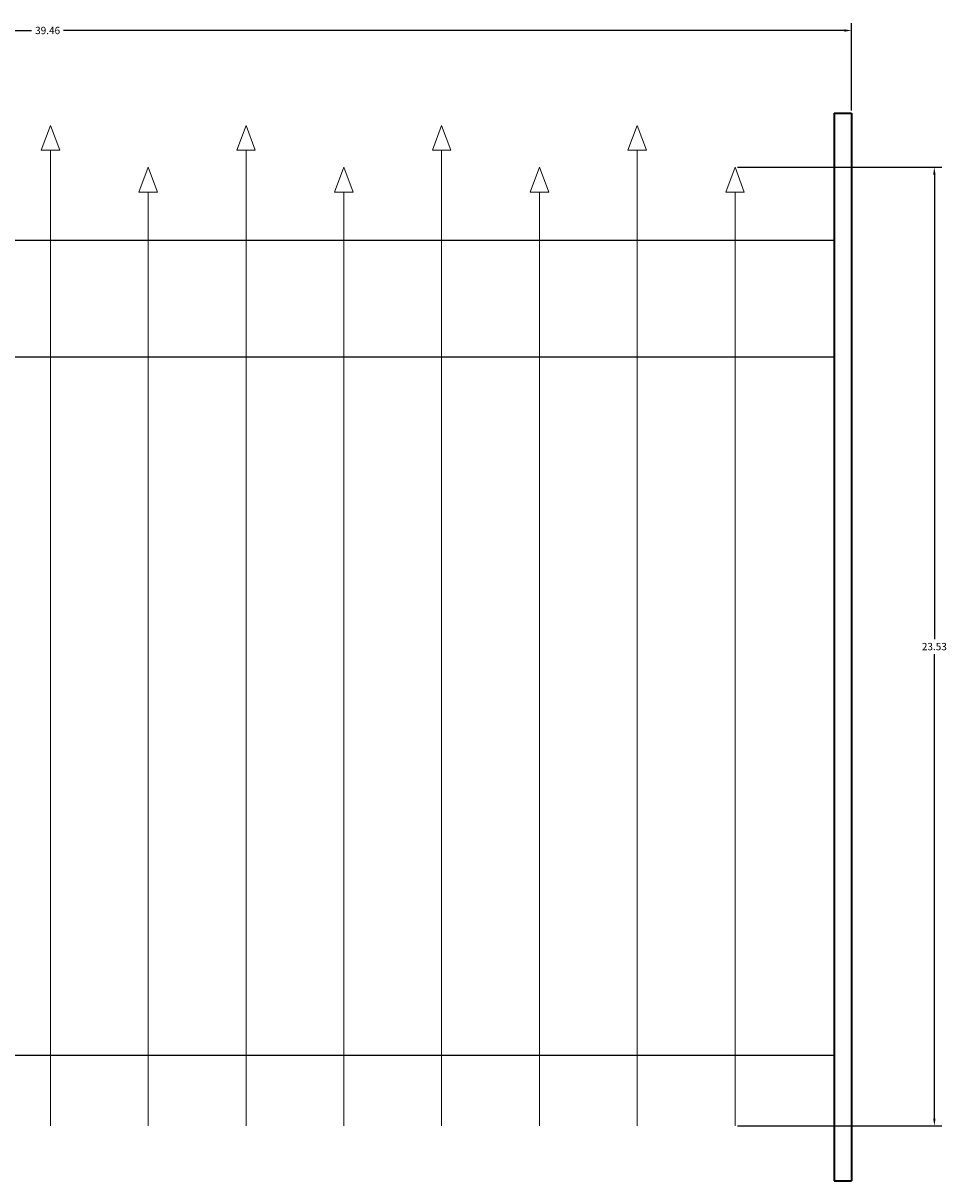
# Model space of a CAD drawing. Units: inches. Extents: x 756 to 915, y 488 to 695.
# Tile 18 of 25: x 789 to 812, y 666 to 694. Entities that reach past the tile are written whole.
import ezdxf

# ---------------------------------------------------------------- set-up
doc = ezdxf.new("R2010")
doc.units = ezdxf.units.IN
doc.header["$MEASUREMENT"] = 0
for name, color, linetype, lineweight in [('L-FENC-PCKT', 7, 'Continuous', 18), ('L-FENC-POST', 7, 'Continuous', 35), ('L-FENC-RAIL', 7, 'Continuous', 25), ('M-DIMS', 2, 'Continuous', 18)]:
    doc.layers.add(name, color=color, linetype=linetype, lineweight=lineweight)
doc.styles.get("Standard").update_dxf_attribs({"font": 'arial.ttf'})
doc.dimstyles.get("Standard").update_dxf_attribs({"dimtxt": 0.18, "dimasz": 0.18, "dimexe": 0.18, "dimexo": 0.0625, "dimgap": 0.09, "dimtad": 0, "dimtih": 1, "dimtoh": 1, "dimdec": 0, "dimzin": 0, "dimdsep": 46, "dimlunit": 3, "dimtxsty": 'Standard', "dimcen": 0.09, "dimadec": 0, "dimazin": 0, "dimtfac": 1, "dimtdec": 0, "dimtofl": 0, "dimtmove": 0, "dimatfit": 3, "dimfxl": 1, "dimtolj": 1, "dimtzin": 0, "dimarcsym": 0})

# ---------------------------------------------------------------- blocks, each defined once
blk = doc.blocks.new('PICKET-SPEAR-EXTENDED')
blk.add_line((0.228, 23.946), (0.228, 0))
blk.add_lwpolyline([(0.228, 23.946), (0, 23.946), (0.228, 24.558), (0.455, 23.946)], close=True)
blk = doc.blocks.new('FENCE-POST-RIGHT')
for p, q in [((0, 26.207), (0, 0)), ((0, 26.207), (0.427, 26.207)), ((0.427, 26.207), (0.427, 0)), ((0, 0), (0.427, 0))]:
    blk.add_line(p, q)
blk = doc.blocks.new('PICKET-SPEAR-LOW')
blk.add_line((0.228, 22.916), (0.228, 0))
blk.add_lwpolyline([(0.228, 22.916), (0, 22.916), (0.228, 23.528), (0.455, 22.916)], close=True)
blk = doc.blocks.new('*D13')
at = {"layer": 'Defpoints', "color": 0, "transparency": 16777216}
for p in [(809.674, 693.983), (770.216, 691.953), (809.674, 691.953)]:
    blk.add_point(p, dxfattribs=at)
at = {"layer": 'M-DIMS', "color": 0, "lineweight": -2, "transparency": 16777216}
for p, q in [((770.216, 692.015), (770.216, 694.163)), ((770.396, 693.983), (789.551, 693.983)), ((809.494, 693.983), (790.338, 693.983)), ((809.674, 692.015), (809.674, 694.163))]:
    blk.add_line(p, q, dxfattribs=at)
at = {"layer": 'M-DIMS', "color": 0, "transparency": 16777216}
for points in [[(770.396, 694.013), (770.396, 693.953), (770.216, 693.983)], [(809.494, 694.013), (809.494, 693.953), (809.674, 693.983)]]:
    blk.add_solid(points, dxfattribs=at)
at = {"layer": 'M-DIMS', "color": 0, "transparency": 16777216, "insert": (789.945, 693.983), "char_height": 0.18, "attachment_point": 5}
blk.add_mtext('\\A1;39.46', dxfattribs=at)
blk = doc.blocks.new('*D17')
at = {"layer": 'Defpoints', "color": 0, "transparency": 16777216}
for p in [(806.814, 690.624), (811.704, 690.624), (806.814, 667.096)]:
    blk.add_point(p, dxfattribs=at)
at = {"layer": 'M-DIMS', "color": 0, "lineweight": -2, "transparency": 16777216}
for p, q in [((806.876, 690.624), (811.884, 690.624)), ((811.704, 690.444), (811.704, 679.042)), ((811.704, 667.276), (811.704, 678.678)), ((806.876, 667.096), (811.884, 667.096))]:
    blk.add_line(p, q, dxfattribs=at)
at = {"layer": 'M-DIMS', "color": 0, "transparency": 16777216}
for points in [[(811.674, 690.444), (811.734, 690.444), (811.704, 690.624)], [(811.674, 667.276), (811.734, 667.276), (811.704, 667.096)]]:
    blk.add_solid(points, dxfattribs=at)
at = {"layer": 'M-DIMS', "color": 0, "transparency": 16777216, "insert": (811.704, 678.86), "char_height": 0.18, "attachment_point": 5}
blk.add_mtext('\\A1;23.53', dxfattribs=at)

msp = doc.modelspace()

# ---------------------------------------------------------------- linework, layer by layer
at = {"layer": 'L-FENC-RAIL'}
for p, q in [((770.6423, 688.8379), (809.2471, 688.8379)), ((770.6423, 685.9735), (809.2471, 685.9735)), ((770.6423, 668.8277), (809.2471, 668.8277))]:
    msp.add_line(p, q, dxfattribs=at)

# ---------------------------------------------------------------- block references
at = {"layer": 'L-FENC-PCKT'}
for name, p in [('PICKET-SPEAR-EXTENDED', (789.7865, 667.096)), ('PICKET-SPEAR-EXTENDED', (794.5863, 667.096)), ('PICKET-SPEAR-EXTENDED', (799.3861, 667.096)), ('PICKET-SPEAR-EXTENDED', (804.1859, 667.096)), ('PICKET-SPEAR-LOW', (792.1863, 667.096)), ('PICKET-SPEAR-LOW', (796.9861, 667.096)), ('PICKET-SPEAR-LOW', (801.7859, 667.096)), ('PICKET-SPEAR-LOW', (806.5858, 667.096))]:
    msp.add_blockref(name, p, dxfattribs=at)
at = {"layer": 'L-FENC-POST'}
msp.add_blockref('FENCE-POST-RIGHT', (809.247, 665.746), dxfattribs=at)

# ---------------------------------------------------------------- dimensions: what is measured, and where the dimension line sits
at = {"layer": 'M-DIMS'}
dim = msp.add_linear_dim(base=(809.6738, 693.9829), p1=(770.2156, 691.9529), p2=(809.6738, 691.9529), dimstyle='Standard', override={"dimdec": 2, "dimlfac": 1, "dimrnd": 0, "dimzin": 0, "dimdsep": 46, "dimlunit": 2}, dxfattribs=at)
dim.commit()
dim.dimension.update_dxf_attribs({"geometry": '*D13', "text_midpoint": (789.9447, 693.9829)})
dim = msp.add_linear_dim(base=(811.7038, 690.6242), p1=(806.8135, 667.0956), p2=(806.8135, 690.6242), angle=90, dimstyle='Standard', override={"dimdec": 2, "dimlfac": 1, "dimrnd": 0, "dimzin": 0, "dimdsep": 46, "dimlunit": 2}, dxfattribs=at)
dim.commit()
dim.dimension.update_dxf_attribs({"geometry": '*D17', "text_midpoint": (811.7038, 678.8599)})

doc.saveas('drawing.dxf')
